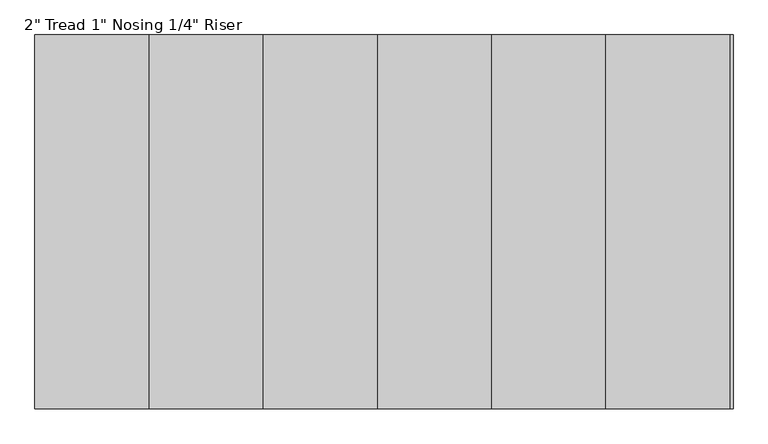
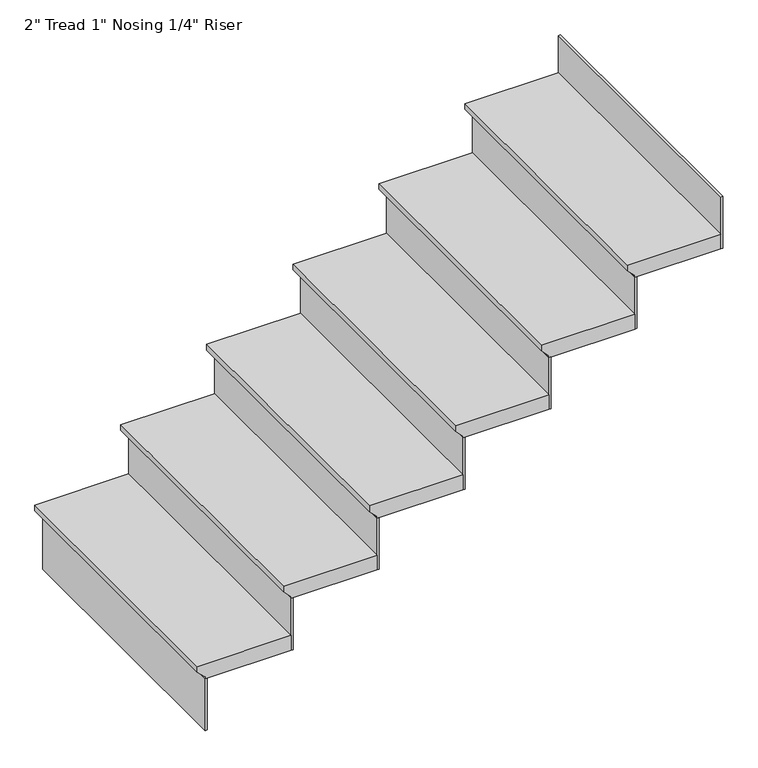
"""IFC4 building model written with IfcOpenShell, lengths in millimetres: stair flight geometry."""

from ifc_helpers import new_model, si_unit, frame, origin, place, context, project, spatial, polyline, outline, extrude, source, transform, mapped, element, save


def stair_flight_2f9793b1(model_context):
    return source(origin(), model_context, "Body", "SweptSolid", [
        extrude(outline(polyline([(5943.6, 20511.9136801), (5943.6, 20207.1136801), (5924.55, 20207.1136801), (5899.15, 20232.5136801), (5892.8, 20232.5136801), (5892.8, 20511.9136801), (5943.6, 20511.9136801)])), frame((0.0, 5614.3752787, 0.0), z_axis=(0.0, 1.0, 0.0), x_axis=(0.0, 0.0, 1.0)), (0.0, 0.0, 1.0), 914.4),
        extrude(outline(polyline([(20238.8636801, 5614.3752787), (20232.5136801, 5614.3752787), (20232.5136801, 6528.7752787), (20238.8636801, 6528.7752787), (20238.8636801, 5614.3752787)])), frame((0.0, 0.0, 5715.0), z_axis=(0.0, 0.0, 1.0), x_axis=(1.0, 0.0, 0.0)), (0.0, 0.0, 1.0), 177.8),
        extrude(outline(polyline([(20518.2636801, 5614.3752787), (20511.9136801, 5614.3752787), (20511.9136801, 6528.7752787), (20518.2636801, 6528.7752787), (20518.2636801, 5614.3752787)])), frame((0.0, 0.0, 5892.8), z_axis=(0.0, 0.0, 1.0), x_axis=(1.0, 0.0, 0.0)), (0.0, 0.0, 1.0), 177.8),
        extrude(outline(polyline([(6121.4, 20791.3136801), (6121.4, 20486.5136801), (6102.35, 20486.5136801), (6076.95, 20511.9136801), (6070.6, 20511.9136801), (6070.6, 20791.3136801), (6121.4, 20791.3136801)])), frame((0.0, 5614.3752787, 0.0), z_axis=(0.0, 1.0, 0.0), x_axis=(0.0, 0.0, 1.0)), (0.0, 0.0, 1.0), 914.4),
        extrude(outline(polyline([(20797.6636801, 5614.3752787), (20791.3136801, 5614.3752787), (20791.3136801, 6528.7752787), (20797.6636801, 6528.7752787), (20797.6636801, 5614.3752787)])), frame((0.0, 0.0, 6070.6), z_axis=(0.0, 0.0, 1.0), x_axis=(1.0, 0.0, 0.0)), (0.0, 0.0, 1.0), 177.8),
        extrude(outline(polyline([(6299.2, 21070.7136801), (6299.2, 20765.9136801), (6280.15, 20765.9136801), (6254.75, 20791.3136801), (6248.4, 20791.3136801), (6248.4, 21070.7136801), (6299.2, 21070.7136801)])), frame((0.0, 5614.3752787, 0.0), z_axis=(0.0, 1.0, 0.0), x_axis=(0.0, 0.0, 1.0)), (0.0, 0.0, 1.0), 914.4),
        extrude(outline(polyline([(21077.0636801, 5614.3752787), (21070.7136801, 5614.3752787), (21070.7136801, 6528.7752787), (21077.0636801, 6528.7752787), (21077.0636801, 5614.3752787)])), frame((0.0, 0.0, 6248.4), z_axis=(0.0, 0.0, 1.0), x_axis=(1.0, 0.0, 0.0)), (0.0, 0.0, 1.0), 177.8),
        extrude(outline(polyline([(6477.0, 21350.1136801), (6477.0, 21045.3136801), (6457.95, 21045.3136801), (6432.55, 21070.7136801), (6426.2, 21070.7136801), (6426.2, 21350.1136801), (6477.0, 21350.1136801)])), frame((0.0, 5614.3752787, 0.0), z_axis=(0.0, 1.0, 0.0), x_axis=(0.0, 0.0, 1.0)), (0.0, 0.0, 1.0), 914.4),
        extrude(outline(polyline([(21356.4636801, 5614.3752787), (21350.1136801, 5614.3752787), (21350.1136801, 6528.7752787), (21356.4636801, 6528.7752787), (21356.4636801, 5614.3752787)])), frame((0.0, 0.0, 6426.2), z_axis=(0.0, 0.0, 1.0), x_axis=(1.0, 0.0, 0.0)), (0.0, 0.0, 1.0), 177.8),
        extrude(outline(polyline([(6654.8, 21629.5136801), (6654.8, 21324.7136801), (6635.75, 21324.7136801), (6610.35, 21350.1136801), (6604.0, 21350.1136801), (6604.0, 21629.5136801), (6654.8, 21629.5136801)])), frame((0.0, 5614.3752787, 0.0), z_axis=(0.0, 1.0, 0.0), x_axis=(0.0, 0.0, 1.0)), (0.0, 0.0, 1.0), 914.4),
        extrude(outline(polyline([(21635.8636801, 5614.3752787), (21629.5136801, 5614.3752787), (21629.5136801, 6528.7752787), (21635.8636801, 6528.7752787), (21635.8636801, 5614.3752787)])), frame((0.0, 0.0, 6604.0), z_axis=(0.0, 0.0, 1.0), x_axis=(1.0, 0.0, 0.0)), (0.0, 0.0, 1.0), 177.8),
        extrude(outline(polyline([(21915.2636801, 5614.3752787), (21908.9136801, 5614.3752787), (21908.9136801, 6528.7752787), (21915.2636801, 6528.7752787), (21915.2636801, 5614.3752787)])), frame((0.0, 0.0, 6781.8), z_axis=(0.0, 0.0, 1.0), x_axis=(1.0, 0.0, 0.0)), (0.0, 0.0, 1.0), 177.8),
        extrude(outline(polyline([(6832.6, 21908.9136801), (6832.6, 21604.1136801), (6813.55, 21604.1136801), (6788.15, 21629.5136801), (6781.8, 21629.5136801), (6781.8, 21908.9136801), (6832.6, 21908.9136801)])), frame((0.0, 5614.3752787, 0.0), z_axis=(0.0, 1.0, 0.0), x_axis=(0.0, 0.0, 1.0)), (0.0, 0.0, 1.0), 914.4),
    ])


if __name__ == "__main__":
    model = new_model("IFC4")
    model_context = context("Model", 3, world=origin())
    ifc_project = project(units=[si_unit("LENGTHUNIT", "METRE", prefix="MILLI")], contexts=[model_context])
    site = spatial("IfcSite", under=ifc_project)
    building = spatial("IfcBuilding", under=site)
    placement = place(None, origin())
    stair_flight_shape = stair_flight_2f9793b1(model_context)
    element("IfcStairFlight", 1, ObjectType="2\" Tread 1\" Nosing 1/4\" Riser", at=placement, inside=building, context=model_context, shape_type="MappedRepresentation", body=[
        mapped(stair_flight_shape, transform((0.0, 0.0, 0.0), x_axis=(1.0, 0.0, 0.0), y_axis=(0.0, 1.0, 0.0), z_axis=(0.0, 0.0, 1.0))),
    ])
    save(model, "model.ifc")
